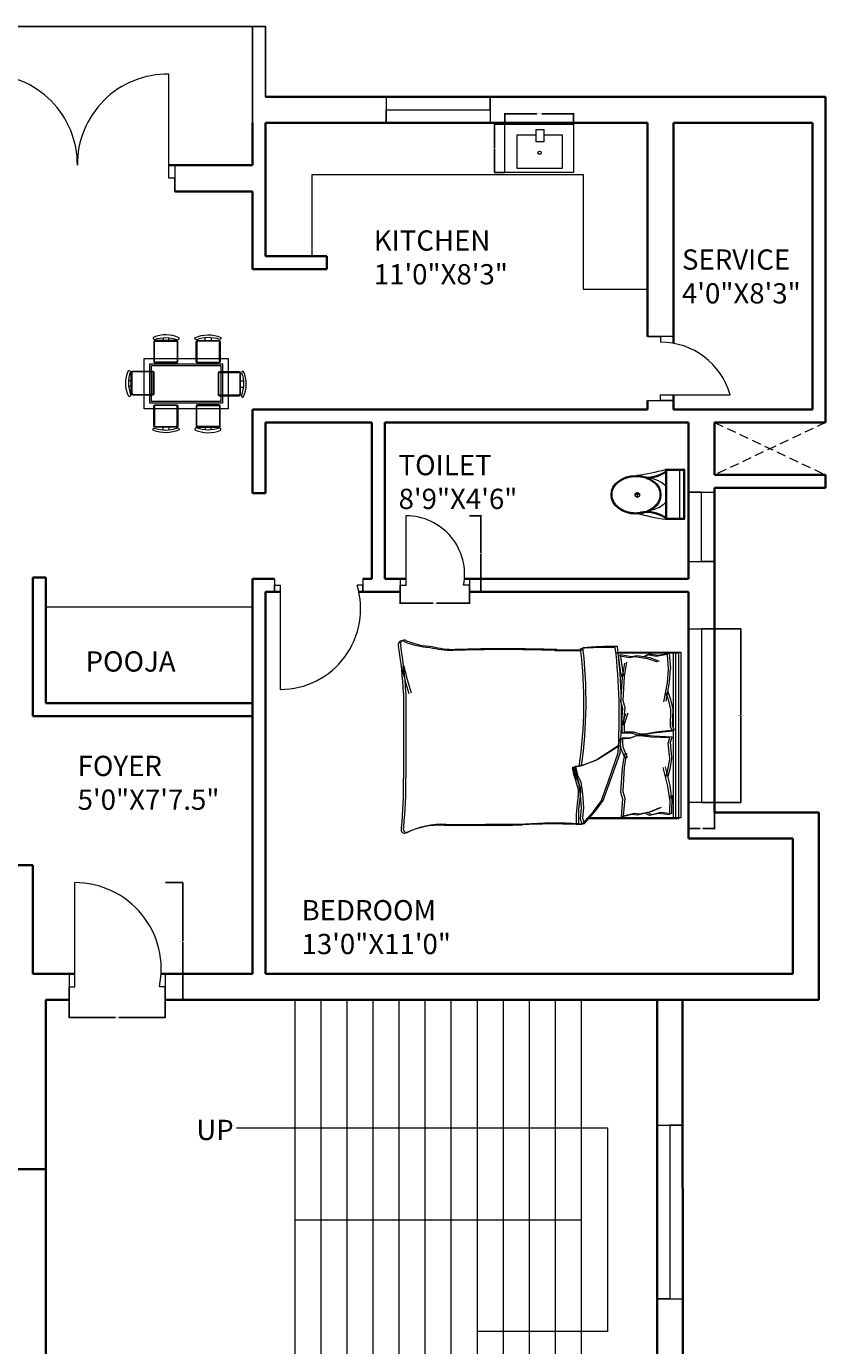
# Model space of a CAD drawing. Units: inches. Extents: x 2296 to 3812, y -1531 to 2564.
# Tile 4 of 10: x 2706 to 2983, y 1719 to 2175. Entities that reach past the tile are written whole.
import ezdxf

# ---------------------------------------------------------------- set-up
doc = ezdxf.new("R2010")
doc.units = ezdxf.units.IN
doc.linetypes.add('HIDDEN2', pattern=[4.7625, 3.175, -1.5875])
for name, color, linetype, lineweight in [('A-ANNO-DIMS', 2, 'Continuous', 18), ('A-ANNO-TEXT', 7, 'Continuous', 25), ('A-AREA-IDEN', 7, 'Continuous', 18), ('A-DOOR', 3, 'Continuous', 18), ('A-FLOR-CASE', 8, 'Continuous', 18), ('A-FLOR-FIXT', 9, 'Continuous', 18), ('A-FLOR-HRAL', 7, 'Continuous', 25), ('A-FLOR-STRS', 7, 'Continuous', 18), ('A-FURN', 8, 'Continuous', 18), ('A-GLAZ', 4, 'Continuous', 18), ('A-WALL', 7, 'Continuous', 35), ('A-WALL-HIDN', 8, 'HIDDEN2', 18)]:
    doc.layers.add(name, color=color, linetype=linetype, lineweight=lineweight)
doc.styles.get("Standard").update_dxf_attribs({"font": 'arial.ttf'})
doc.dimstyles.get("Standard").update_dxf_attribs({"dimtxt": 0.18, "dimasz": 0.18, "dimexe": 0.18, "dimexo": 0.0625, "dimgap": 0.09, "dimtad": 0, "dimtih": 1, "dimtoh": 1, "dimdec": 4, "dimzin": 0, "dimdsep": 46, "dimtxsty": 'Standard', "dimcen": 0.09, "dimadec": 0, "dimazin": 0, "dimtfac": 1, "dimtdec": 4, "dimtofl": 0, "dimtmove": 0, "dimatfit": 3, "dimfxl": 1, "dimtolj": 1, "dimtzin": 0, "dimarcsym": 0})

# ---------------------------------------------------------------- blocks, each defined once
blk = doc.blocks.new('A$C31115884')
for p, q in [((283, 498), (223, 498)), ((258, 466), (258, 523)), ((0, 200), (0, 0)), ((520, 200), (0, 200)), ((10, 190), (10, 10)), ((510, 190), (10, 190)), ((510, 10), (510, 190)), ((520, 0), (520, 200)), ((510, 54), (0, 54)), ((10, 10), (510, 10)), ((0, 0), (520, 0))]:
    blk.add_line(p, q)
blk.add_circle((256, 496), 23.6)
for centre, radius, start, end in [((2778, -205), 2807, 165.4549, 171.7133), ((-295, 403), 365, 324.2091, 9.3499), ((-295, 403), 375, 324.2091, 9.3499), ((139, 406), 293, 315.8436, 2.6563), ((806, 403), 365, 170.6501, 215.7909), ((3237, 905), 2807, 188.2867, 194.5451), ((384, 406), 293, 190.2774, 224.1564), ((806, 403), 375, 179.2036, 215.7909)]:
    blk.add_arc(centre, radius, start, end)
blk.add_ellipse((256, 510), major_axis=(0, -261), ratio=0.772727)
blk.add_open_spline([(256, 259), (263, 259), (270, 260), (288, 262), (299, 265), (320, 273), (330, 278), (350, 291), (360, 299), (378, 316), (386, 326), (402, 347), (409, 358), (421, 383), (427, 395), (436, 422), (440, 436), (445, 465), (447, 480), (448, 509), (448, 524), (445, 553), (443, 568), (436, 596), (432, 610), (422, 636), (416, 649), (402, 672), (395, 683), (379, 703), (370, 712), (351, 728), (341, 735), (321, 746), (310, 751), (289, 757), (278, 759), (256, 761), (245, 761), (223, 757), (212, 754), (191, 746), (181, 741), (161, 728), (151, 720), (133, 703), (125, 693), (110, 672), (103, 660), (90, 636), (85, 623), (76, 596), (72, 582), (67, 553), (66, 538), (64, 509), (65, 494), (68, 465), (70, 450), (77, 422), (81, 408), (91, 382), (97, 370), (111, 346), (118, 335), (135, 316), (144, 307), (162, 291), (172, 284), (193, 273), (203, 269), (225, 262), (236, 260), (250, 259), (253, 259), (256, 259)], degree=3, knots=[0, 0, 0, 0, 0.110105, 0.110105, 0.285049, 0.285049, 0.459994, 0.459994, 0.634938, 0.634938, 0.809882, 0.809882, 0.984827, 0.984827, 1.159771, 1.159771, 1.334715, 1.334715, 1.50966, 1.50966, 1.684604, 1.684604, 1.859549, 1.859549, 2.034493, 2.034493, 2.209437, 2.209437, 2.384382, 2.384382, 2.559326, 2.559326, 2.73427, 2.73427, 2.909215, 2.909215, 3.084159, 3.084159, 3.259103, 3.259103, 3.434048, 3.434048, 3.608992, 3.608992, 3.783936, 3.783936, 3.958881, 3.958881, 4.133825, 4.133825, 4.30877, 4.30877, 4.483714, 4.483714, 4.658658, 4.658658, 4.833603, 4.833603, 5.008547, 5.008547, 5.183491, 5.183491, 5.358436, 5.358436, 5.53338, 5.53338, 5.708324, 5.708324, 5.883269, 5.883269, 6.058213, 6.058213, 6.233158, 6.233158, 6.283185, 6.283185, 6.283185, 6.283185])
blk = doc.blocks.new('DOOR-SERVICE-24-NE')
for p, q in [((9, 22.16), (0, 22.16)), ((0, 22.16), (4.5, 22.16)), ((4.5, 22.16), (4.5, 20.16)), ((0, 0), (9, 0)), ((4.5, 0), (4.5, 2)), ((4.5, 2), (28.5, 2)), ((9, 0), (4.5, 0))]:
    blk.add_line(p, q)
blk.add_arc((4.5, -4.78), 24.94, 15.78, 90)
blk = doc.blocks.new('DOOR-BALCONY-PAIR-N')
for p, q in [((2, 4.5), (2, 40.5)), ((64.91, 4.5), (64.91, 40.5)), ((0, 9), (0, 0)), ((66.91, 9), (66.91, 0)), ((0, 0), (0, 4.5)), ((0, 4.5), (2, 4.5)), ((66.91, 4.5), (64.91, 4.5)), ((66.91, 0), (66.91, 4.5))]:
    blk.add_line(p, q)
for centre, radius, start, end in [((2, 9.22), 31.28, 359.5901, 90), ((64.41, 9.36), 31.14, 89.0831, 180.6679)]:
    blk.add_arc(centre, radius, start, end)
blk = doc.blocks.new('DOOR-BEDROOM-36-NE')
for p, q in [((0, 38.25), (0, 33.75)), ((30.56, 38.25), (30.56, 33.75)), ((0, 33.75), (0, 36)), ((0, 36), (0, 36)), ((0, 36), (2, 36)), ((2, 36), (2, 0)), ((30.56, 36), (28.56, 36)), ((30.56, 33.75), (30.56, 36))]:
    blk.add_line(p, q)
blk.add_arc((2, 27.8), 27.8, 270, 17.157)
blk = doc.blocks.new('DOOR-BATH-24-NE')
for p, q in [((2, 2.25), (2, 26.25)), ((0, 4.5), (0, 0)), ((0, 0), (0, 2.25)), ((0, 2.25), (2, 2.25)), ((23.89, 2.25), (21.89, 2.25)), ((23.89, 4.5), (23.89, 0)), ((23.89, 0), (23.89, 2.25))]:
    blk.add_line(p, q)
blk.add_arc((2, 6.01), 20.24, 349.2884, 90)
blk = doc.blocks.new('DOOR-ENTRY-36-N')
for p, q in [((2, 4.5), (2, 40.5)), ((0, 9), (0, 0)), ((33.22, 9), (33.22, 0)), ((0, 0), (0, 4.5)), ((0, 4.5), (2, 4.5)), ((33.22, 4.5), (31.22, 4.5)), ((33.22, 0), (33.22, 4.5))]:
    blk.add_line(p, q)
blk.add_arc((2, 10.64), 29.86, 348.1386, 90)
blk = doc.blocks.new('WIN-36-KITCHEN')
for p, q in [((0, 9), (0, 0)), ((36, 4.5), (36, 9)), ((36, 9), (36, 0)), ((0, 0), (0, 4.5)), ((0, 4.5), (36, 4.5))]:
    blk.add_line(p, q)
blk = doc.blocks.new('WIN-24-BATH')
for p, q in [((4.5, 24), (0, 24)), ((0, 24), (9, 24)), ((4.5, 0), (4.5, 24)), ((0, 0), (9, 0)), ((9, 0), (4.5, 0))]:
    blk.add_line(p, q)
blk = doc.blocks.new('WIN-60-JAMB-A')
for p, q in [((0, 60), (9, 60)), ((9, 60), (4.5, 60)), ((4.5, 60), (4.5, 0)), ((9, 0), (0, 0)), ((4.5, 0), (9, 0))]:
    blk.add_line(p, q)
blk = doc.blocks.new('WIN-60-STAIR')
for p, q in [((0, 59.99), (8.73, 60.01)), ((8.73, 60.01), (4.36, 60)), ((4.36, 60), (4.36, 0)), ((0, 0), (8.81, 0.01)), ((4.36, 0), (0, 0))]:
    blk.add_line(p, q)
blk = doc.blocks.new('BED-DOUBLE')
for p, q in [((48.49, 95), (18.98, 95)), ((3.07, 35.36), (3.17, 33.26, 4.64)), ((5.01, 34.01), (3.17, 33.26)), ((3.17, 33.26), (7.61, 29.37)), ((8.72, 33.63), (5.01, 34.01)), ((13.37, 34.01), (8.72, 33.63)), ((17.45, 34.56), (13.37, 34.01)), ((19.86, 35.68), (17.45, 34.56)), ((22.83, 36.42), (19.86, 35.68)), ((23.21, 34.01), (22.83, 36.42)), ((25.25, 28.62), (23.21, 34.01)), ((5.09, 0), (5.09, 31.9)), ((7.61, 29.37), (11.14, 26.77)), ((30.27, 20.84), (25.25, 28.62)), ((11.14, 26.77), (17.82, 24.36)), ((17.82, 24.36), (27.82, 20.84)), ((11.92, 19.38), (5.77, 19.87)), ((5.77, 19.87), (6.7, 16.11)), ((14.27, 20.05), (11.92, 19.38)), ((22.67, 19.54), (14.27, 20.05)), ((27.51, 18.74), (22.67, 19.54)), ((29.68, 20.07), (26, 18.53)), ((32.62, 20.25), (29.68, 20.07)), ((32.82, 17.04), (32.62, 20.25)), ((34.71, 16.28), (34.71, 19.5)), ((34.71, 19.5), (37.65, 19.5)), ((43.31, 19.38), (37.16, 19.87)), ((37.65, 19.5), (41.42, 18.19)), ((45.66, 20.05), (43.31, 19.38)), ((54.06, 19.54), (45.66, 20.05)), ((54.06, 19.54), (55.42, 19.92)), ((58.9, 18.74), (54.06, 19.54)), ((55.42, 19.92), (61.53, 20.79)), ((61.53, 20.79), (60.84, 16.98)), ((62.38, 21.71), (62.38, 0)), ((6.7, 16.11), (6.47, 14.18)), ((6.47, 14.18), (7.43, 9.9)), ((33.66, 14.84), (32.82, 17.04)), ((33.75, 13.28), (33.66, 14.84)), ((34.01, 14.03), (34.71, 16.28)), ((34.01, 12.47), (34.01, 14.03)), ((61.19, 15.07), (60.49, 10.74)), ((60.84, 16.98), (61.19, 15.07)), ((6.21, 10), (6.83, 11.25)), ((6.93, 6.92), (6.21, 10)), ((7.43, 9.9), (8.85, 6.69)), ((33.01, 2.99), (33.3, 9.43)), ((33.3, 9.43), (33.75, 13.28)), ((34.71, 8.66), (34.01, 12.47)), ((60.49, 10.74), (59.28, 7.44)), ((61.71, 10.91), (61.01, 12.12)), ((61.19, 7.79), (61.71, 10.91)), ((6.47, 3.07), (6.93, 6.92)), ((16.3, 3.68), (22.8, 5.3)), ((35.4, 2.24), (34.71, 8.66)), ((52.03, 3.98), (45.45, 5.19)), ((61.88, 3.98), (61.19, 7.79)), ((62.38, 1.84), (5.09, 1.84)), ((62.38, 0), (5.09, 0)), ((6.47, 3.07), (12.95, 2.95)), ((11.75, 3.05), (16.3, 3.68)), ((12.95, 2.95), (11.75, 3.05)), ((19.55, 4.4), (22.03, 3.69)), ((22.03, 3.69), (25.54, 3.04)), ((25.54, 3.04), (25.93, 3.07)), ((25.93, 3.07), (31.24, 3.57)), ((31.24, 3.57), (33.01, 2.99)), ((37.13, 2.94), (35.4, 2.24)), ((42.46, 2.76), (37.13, 2.94)), ((42.85, 2.76), (42.46, 2.76)), ((46.31, 3.63), (42.85, 2.76)), ((48.74, 4.5), (46.31, 3.63)), ((56.62, 3.63), (52.03, 3.98)), ((56.74, 3.61), (56.62, 3.63)), ((61.87, 4), (56.74, 3.61))]:
    blk.add_line(p, q)
for centre, radius, start, end in [((1.32, 94.55), 1.32, 62.6588, 176.02), ((87.19, -28.43), 127.63, 103.3832, 107.7053), ((40.86, 240.78), 145.97, 272.9958, 279.4091), ((65.24, 95.57), 1.31, 326.1736, 113.4781), ((-24.75, 82.32), 27.65, 357.4714, 26.4681), ((17.21, 254.49), 159.5, 264.4998, 270.6351), ((92.52, 84.25), 28.25, 157.9751, 176.652), ((98.8, 77.34), 35.53, 166.0648, 178.9113), ((5471.89, 81.31), 5469.02, 180.00217, 180.28689), ((-514.68, 60.68), 578.22, 358.22771, 1.71854), ((-151.96, 43.54), 155.25, 356.9791, 3.8365), ((267.13, 37.37), 203.94, 178.4762, 181.0082), ((29.2, 1.78), 35.55, 100.6617, 109.8806), ((22.63, 36.49), 0.221, 340.2464, 91.1377), ((5.01, -7.98), 43.38, 79.8763, 92.5657), ((14.11, 42.04), 7.46, 258.6608, 293.7384), ((45.26, 187.4), 154.68, 261.7845, 276.9006), ((-35.55, 24.09), 99.87, 358.7218, 5.604), ((40.94, 218.26), 197.77, 266.0865, 276.7821)]:
    blk.add_arc(centre, radius, start, end)
blk = doc.blocks.new('SINK-KITCHEN')
for points in [[(0, 16.77), (23.71, 16.77), (23.71, 0), (0, 0)], [(10.76, 14.92), (13.44, 14.92), (13.44, 10.63), (10.76, 10.63)]]:
    blk.add_lwpolyline(points, close=True)
blk.add_lwpolyline([(13.44, 13.06), (19.73, 13.06), (19.73, 1.48), (4.23, 1.48), (4.23, 13.06), (10.76, 13.06)])
blk.add_circle((11.97, 6.87), 0.556)
blk = doc.blocks.new('STAIR-DOGLEG')
for p, q in [((20.27, 0), (20.27, 152.06)), ((29.27, 0), (29.27, 152.06)), ((38.27, 0), (38.27, 152.06)), ((47.27, 0), (47.27, 152.06)), ((56.27, 0), (56.27, 152.06)), ((65.27, 0), (65.27, 152.06)), ((74.27, 0), (74.27, 152.06)), ((83.27, 0), (83.27, 152.06)), ((92.27, 0), (92.27, 152.06)), ((101.27, 0), (101.27, 152.06)), ((110.27, 0), (110.27, 152.06)), ((119.27, 0), (119.27, 152.06)), ((0, 107.85), (128.27, 107.85)), ((128.27, 107.85), (128.27, 37.4)), ((20.27, 76.03), (119.27, 76.03)), ((128.27, 37.4), (83.27, 37.4))]:
    blk.add_line(p, q)
blk = doc.blocks.new('COUNTER-KITCHEN-N')
for p, q in [((0, 11.4), (0, 39.66)), ((0, 39.66), (93.66, 39.66)), ((93.66, 39.66), (93.66, 0)), ((93.66, 0), (115.91, 0))]:
    blk.add_line(p, q)
blk = doc.blocks.new('*D47')
at = {"layer": 'A-ANNO-DIMS', "color": 0, "lineweight": -2, "transparency": 16777216}
for p, q in [((2871.76, 2141.32), (2871.76, 2144.99)), ((2871.94, 2144.81), (2882.76, 2144.81)), ((2895.29, 2144.81), (2884.47, 2144.81)), ((2895.47, 2141.32), (2895.47, 2144.99))]:
    blk.add_line(p, q, dxfattribs=at)
at = {"layer": 'A-ANNO-DIMS', "color": 0, "transparency": 16777216}
for points in [[(2871.94, 2144.84), (2871.94, 2144.78), (2871.76, 2144.81)], [(2895.29, 2144.84), (2895.29, 2144.78), (2895.47, 2144.81)]]:
    blk.add_solid(points, dxfattribs=at)
at = {"layer": 'Defpoints', "color": 0, "transparency": 16777216}
for p in [(2895.47, 2144.81), (2871.76, 2141.25), (2895.47, 2141.25)]:
    blk.add_point(p, dxfattribs=at)
at = {"layer": 'A-ANNO-DIMS', "color": 0, "transparency": 16777216, "insert": (2883.61, 2144.81), "char_height": 0.18, "attachment_point": 5}
blk.add_mtext('\\A1;SINK 24 TYP.', dxfattribs=at)
blk = doc.blocks.new('*D48')
at = {"layer": 'A-ANNO-DIMS', "color": 0, "lineweight": -2, "transparency": 16777216}
for p, q in [((2871.7, 2141.25), (2868.02, 2141.25)), ((2868.2, 2141.07), (2868.2, 2133.05)), ((2868.2, 2124.66), (2868.2, 2132.69)), ((2871.7, 2124.48), (2868.02, 2124.48))]:
    blk.add_line(p, q, dxfattribs=at)
at = {"layer": 'A-ANNO-DIMS', "color": 0, "transparency": 16777216}
for points in [[(2868.17, 2141.07), (2868.23, 2141.07), (2868.2, 2141.25)], [(2868.17, 2124.66), (2868.23, 2124.66), (2868.2, 2124.48)]]:
    blk.add_solid(points, dxfattribs=at)
at = {"layer": 'Defpoints', "color": 0, "transparency": 16777216}
for p in [(2868.2, 2141.25), (2871.76, 2141.25), (2871.76, 2124.48)]:
    blk.add_point(p, dxfattribs=at)
at = {"layer": 'A-ANNO-DIMS', "color": 0, "transparency": 16777216, "insert": (2868.2, 2132.87), "char_height": 0.18, "attachment_point": 5}
blk.add_mtext('\\A1;17 TYP.', dxfattribs=at)
blk = doc.blocks.new('*D67')
at = {"layer": 'A-ANNO-DIMS', "color": 0, "lineweight": -2, "transparency": 16777216}
for p, q in [((2859.56, 2005.91), (2863.62, 2005.91)), ((2863.44, 2005.73), (2863.44, 1992.97)), ((2863.44, 1979.84), (2863.44, 1992.6)), ((2859.56, 1979.66), (2863.62, 1979.66))]:
    blk.add_line(p, q, dxfattribs=at)
at = {"layer": 'A-ANNO-DIMS', "color": 0, "transparency": 16777216}
for points in [[(2863.41, 2005.73), (2863.47, 2005.73), (2863.44, 2005.91)], [(2863.41, 1979.84), (2863.47, 1979.84), (2863.44, 1979.66)]]:
    blk.add_solid(points, dxfattribs=at)
at = {"layer": 'Defpoints', "color": 0, "transparency": 16777216}
for p in [(2859.5, 2005.91), (2863.44, 2005.91), (2859.5, 1979.66)]:
    blk.add_point(p, dxfattribs=at)
at = {"layer": 'A-ANNO-DIMS', "color": 0, "transparency": 16777216, "insert": (2863.44, 1992.78), "char_height": 0.18, "attachment_point": 5}
blk.add_mtext('\\A1;BATH DOOR 26 TYP.', dxfattribs=at)
blk = doc.blocks.new('*D68')
at = {"layer": 'A-ANNO-DIMS', "color": 0, "lineweight": -2, "transparency": 16777216}
for p, q in [((2835.61, 1979.6), (2835.61, 1975.54)), ((2859.5, 1979.6), (2859.5, 1975.54)), ((2835.79, 1975.72), (2847.03, 1975.72)), ((2859.32, 1975.72), (2848.09, 1975.72))]:
    blk.add_line(p, q, dxfattribs=at)
at = {"layer": 'A-ANNO-DIMS', "color": 0, "transparency": 16777216}
for points in [[(2835.79, 1975.75), (2835.79, 1975.69), (2835.61, 1975.72)], [(2859.32, 1975.75), (2859.32, 1975.69), (2859.5, 1975.72)]]:
    blk.add_solid(points, dxfattribs=at)
at = {"layer": 'Defpoints', "color": 0, "transparency": 16777216}
for p in [(2835.61, 1979.66), (2859.5, 1979.66), (2859.5, 1975.72)]:
    blk.add_point(p, dxfattribs=at)
at = {"layer": 'A-ANNO-DIMS', "color": 0, "transparency": 16777216, "insert": (2847.56, 1975.72), "char_height": 0.18, "attachment_point": 5}
blk.add_mtext('\\A1;24 TYP.', dxfattribs=at)
blk = doc.blocks.new('*D73')
at = {"layer": 'A-ANNO-DIMS', "color": 0, "lineweight": -2, "transparency": 16777216}
for p, q in [((2754.46, 1879.16), (2760.65, 1879.16)), ((2760.47, 1878.98), (2760.47, 1859.09)), ((2760.47, 1838.84), (2760.47, 1858.72)), ((2754.46, 1838.66), (2760.65, 1838.66))]:
    blk.add_line(p, q, dxfattribs=at)
at = {"layer": 'A-ANNO-DIMS', "color": 0, "transparency": 16777216}
for points in [[(2760.44, 1878.98), (2760.5, 1878.98), (2760.47, 1879.16)], [(2760.44, 1838.84), (2760.5, 1838.84), (2760.47, 1838.66)]]:
    blk.add_solid(points, dxfattribs=at)
at = {"layer": 'Defpoints', "color": 0, "transparency": 16777216}
for p in [(2754.39, 1879.16), (2760.47, 1879.16), (2754.39, 1838.66)]:
    blk.add_point(p, dxfattribs=at)
at = {"layer": 'A-ANNO-DIMS', "color": 0, "transparency": 16777216, "insert": (2760.47, 1858.91), "char_height": 0.18, "attachment_point": 5}
blk.add_mtext('\\A1;ENTRY DOOR 41 TYP.', dxfattribs=at)
blk = doc.blocks.new('*D74')
at = {"layer": 'A-ANNO-DIMS', "color": 0, "lineweight": -2, "transparency": 16777216}
for p, q in [((2721.17, 1838.6), (2721.17, 1832.4)), ((2754.39, 1838.6), (2754.39, 1832.4)), ((2721.35, 1832.58), (2737.25, 1832.58)), ((2754.21, 1832.58), (2738.31, 1832.58))]:
    blk.add_line(p, q, dxfattribs=at)
at = {"layer": 'A-ANNO-DIMS', "color": 0, "transparency": 16777216}
for points in [[(2721.35, 1832.61), (2721.35, 1832.55), (2721.17, 1832.58)], [(2754.21, 1832.61), (2754.21, 1832.55), (2754.39, 1832.58)]]:
    blk.add_solid(points, dxfattribs=at)
at = {"layer": 'Defpoints', "color": 0, "transparency": 16777216}
for p in [(2721.17, 1838.66), (2754.39, 1838.66), (2754.39, 1832.58)]:
    blk.add_point(p, dxfattribs=at)
at = {"layer": 'A-ANNO-DIMS', "color": 0, "transparency": 16777216, "insert": (2737.78, 1832.58), "char_height": 0.18, "attachment_point": 5}
blk.add_mtext('\\A1;33 TYP.', dxfattribs=at)
blk = doc.blocks.new('*D95')
at = {"layer": 'A-ANNO-DIMS', "color": 0, "lineweight": -2, "transparency": 16777216}
for p, q in [((2944.29, 1966.83), (2953.41, 1966.83)), ((2953.23, 1966.65), (2953.23, 1937.01)), ((2953.23, 1907.01), (2953.23, 1936.65)), ((2944.29, 1906.83), (2953.41, 1906.83))]:
    blk.add_line(p, q, dxfattribs=at)
at = {"layer": 'A-ANNO-DIMS', "color": 0, "transparency": 16777216}
for points in [[(2953.2, 1966.65), (2953.26, 1966.65), (2953.23, 1966.83)], [(2953.2, 1907.01), (2953.26, 1907.01), (2953.23, 1906.83)]]:
    blk.add_solid(points, dxfattribs=at)
at = {"layer": 'Defpoints', "color": 0, "transparency": 16777216}
for p in [(2944.23, 1966.83), (2953.23, 1966.83), (2944.23, 1906.83)]:
    blk.add_point(p, dxfattribs=at)
at = {"layer": 'A-ANNO-DIMS', "color": 0, "transparency": 16777216, "insert": (2953.23, 1936.83), "char_height": 0.18, "attachment_point": 5}
blk.add_mtext('\\A1;WINDOW 60 TYP.', dxfattribs=at)
blk = doc.blocks.new('*D96')
at = {"layer": 'A-ANNO-DIMS', "color": 0, "lineweight": -2, "transparency": 16777216}
for p, q in [((2935.23, 1906.77), (2935.23, 1897.65)), ((2944.23, 1906.77), (2944.23, 1897.65)), ((2935.41, 1897.83), (2939.27, 1897.83)), ((2944.05, 1897.83), (2940.19, 1897.83))]:
    blk.add_line(p, q, dxfattribs=at)
at = {"layer": 'A-ANNO-DIMS', "color": 0, "transparency": 16777216}
for points in [[(2935.41, 1897.86), (2935.41, 1897.8), (2935.23, 1897.83)], [(2944.05, 1897.86), (2944.05, 1897.8), (2944.23, 1897.83)]]:
    blk.add_solid(points, dxfattribs=at)
at = {"layer": 'Defpoints', "color": 0, "transparency": 16777216}
for p in [(2935.23, 1906.83), (2944.23, 1906.83), (2944.23, 1897.83)]:
    blk.add_point(p, dxfattribs=at)
at = {"layer": 'A-ANNO-DIMS', "color": 0, "transparency": 16777216, "insert": (2939.73, 1897.83), "char_height": 0.18, "attachment_point": 5}
blk.add_mtext('\\A1;9 TYP.', dxfattribs=at)

msp = doc.modelspace()

# ---------------------------------------------------------------- linework, layer by layer
at = {"layer": 'A-FLOR-CASE'}
msp.add_line((2784.5693, 1974.3293), (2713.1754, 1974.3293), dxfattribs=at)
at = {"layer": 'A-FLOR-HRAL'}
for p, q in [((2789.0693, 2175.0276), (2655.5693, 2175.0276)), ((2660.0693, 2175.0276), (2789.0693, 2175.0276)), ((2784.5693, 2141.6578), (2784.5693, 2175.0276)), ((2789.0693, 2175.0276), (2789.0693, 2150.6578))]:
    msp.add_line(p, q, dxfattribs=at)
at = {"layer": 'A-FURN'}
for points in [[(2750.6939, 2066.831, -0.17580919), (2758.5956, 2066.7712, 0.57839206), (2759.1942, 2067.4294, 0.21452438), (2750.2749, 2067.5491, 0.55201397), (2750.6939, 2066.831, -0.06507904)], [(2758.2603, 2066.5139), (2750.9247, 2066.5139, 0.41421356), (2750.4115, 2066.0007), (2750.4115, 2059.2556, 0.41421356), (2750.9247, 2058.7424), (2758.2603, 2058.7424, 0.41421356), (2758.7736, 2059.2556), (2758.7736, 2066.0007, 0.41421356), (2758.2603, 2066.5139)], [(2755.6837, 2066.5139), (2755.6837, 2067.4416, -0.06475861)], [(2765.2478, 2066.7712, -0.57839206), (2764.6492, 2067.4294, -0.21452438), (2773.5685, 2067.5491, -0.55201397), (2773.1495, 2066.831, 0.1758092), (2765.2478, 2066.7712)], [(2772.9187, 2066.5139, -0.41421356), (2773.4319, 2066.0007), (2773.4319, 2059.2556, -0.41421356), (2772.9187, 2058.7424), (2765.583, 2058.7424, -0.41421356), (2765.0698, 2059.2556), (2765.0698, 2066.0007, -0.41421356), (2765.583, 2066.5139), (2772.9187, 2066.5139)], [(2768.1597, 2066.5139), (2768.1597, 2067.4416, 0.06475861)], [(2742.4272, 2047.7496, -0.57839206), (2741.769, 2047.151, -0.21452438), (2741.6493, 2056.0703, -0.55201397), (2742.3673, 2055.6513, 0.17580937), (2742.4272, 2047.7496)], [(2742.6845, 2055.4205, -0.41421356), (2743.1977, 2055.9337), (2749.9427, 2055.9337, -0.41421356), (2750.4559, 2055.4205), (2750.4559, 2048.0848, -0.41421356), (2749.9427, 2047.5716), (2743.1977, 2047.5716, -0.41421356), (2742.6845, 2048.0848), (2742.6845, 2055.4205)], [(2780.4598, 2055.1693, 0.41421356), (2779.9466, 2055.6825), (2773.2015, 2055.6825, 0.41421356), (2772.6883, 2055.1693), (2772.6883, 2047.8336, 0.41421356), (2773.2015, 2047.3204), (2779.9466, 2047.3204, 0.41421356), (2780.4598, 2047.8336), (2780.4598, 2055.1693)], [(2780.7769, 2055.4001, -0.17580919), (2780.7171, 2047.4984, 0.57839206), (2781.3753, 2046.8997, 0.21452438), (2781.495, 2055.8191, 0.55201397), (2780.7769, 2055.4001, -0.06507904)], [(2742.6845, 2050.6615), (2741.7567, 2050.6615, 0.06475861)], [(2780.4598, 2050.4103), (2781.3875, 2050.4103, -0.06475861)], [(2758.2603, 2036.5306), (2750.9247, 2036.5306, -0.41421356), (2750.4115, 2037.0439), (2750.4115, 2043.7889, -0.41421356), (2750.9247, 2044.3021), (2758.2603, 2044.3021, -0.41421356), (2758.7736, 2043.7889), (2758.7736, 2037.0439, -0.41421356), (2758.2603, 2036.5306)], [(2772.9187, 2036.5306, 0.41421356), (2773.4319, 2037.0439), (2773.4319, 2043.7889, 0.41421356), (2772.9187, 2044.3021), (2765.583, 2044.3021, 0.41421356), (2765.0698, 2043.7889), (2765.0698, 2037.0439, 0.41421356), (2765.583, 2036.5306), (2772.9187, 2036.5306)], [(2758.5956, 2036.2733, -0.57839206), (2759.1942, 2035.6151, -0.21452438), (2750.2749, 2035.4954, -0.55201397), (2750.6939, 2036.2135, 0.17580929), (2758.5956, 2036.2733)], [(2755.6837, 2036.5306), (2755.6837, 2035.6029, 0.06475861)], [(2773.1495, 2036.2135, -0.17580928), (2765.2478, 2036.2733, 0.57839206), (2764.6492, 2035.6151, 0.21452438), (2773.5685, 2035.4954, 0.55201397), (2773.1495, 2036.2135, -0.06507904)], [(2768.1597, 2036.5306), (2768.1597, 2035.6029, -0.06475861)]]:
    msp.add_lwpolyline(points, format="xyb", dxfattribs=at)
for points in [[(2750.9278, 2066.2827), (2758.0291, 2066.2827, -0.41421356), (2758.5424, 2065.7694), (2758.5424, 2059.4868, -0.41421356), (2758.0291, 2058.9736), (2750.9278, 2058.9736, -0.51206948), (2750.6427, 2059.4868), (2750.6427, 2065.7694, -0.51206948)], [(2772.9156, 2066.2827), (2765.8142, 2066.2827, 0.41421356), (2765.301, 2065.7694), (2765.301, 2059.4868, 0.41421356), (2765.8142, 2058.9736), (2772.9156, 2058.9736, 0.51206948), (2773.2007, 2059.4868), (2773.2007, 2065.7694, 0.51206948)], [(2742.9157, 2055.4174), (2742.9157, 2048.316, 0.41421356), (2743.4289, 2047.8028), (2749.7115, 2047.8028, 0.41421356), (2750.2247, 2048.316), (2750.2247, 2055.4174, 0.51206948), (2749.7115, 2055.7025), (2743.4289, 2055.7025, 0.51206948)], [(2780.2286, 2055.1662), (2780.2286, 2048.0648, -0.41421356), (2779.7154, 2047.5516), (2773.4328, 2047.5516, -0.41421356), (2772.9195, 2048.0648), (2772.9195, 2055.1662, -0.51206948), (2773.4328, 2055.4513), (2779.7154, 2055.4513, -0.51206948)], [(2750.9278, 2036.7618), (2758.0291, 2036.7618, 0.41421356), (2758.5424, 2037.2751), (2758.5424, 2043.5577, 0.41421356), (2758.0291, 2044.0709), (2750.9278, 2044.0709, 0.51206948), (2750.6427, 2043.5577), (2750.6427, 2037.2751, 0.51206948)], [(2772.9156, 2036.7618), (2765.8142, 2036.7618, -0.41421356), (2765.301, 2037.2751), (2765.301, 2043.5577, -0.41421356), (2765.8142, 2044.0709), (2772.9156, 2044.0709, -0.51206948), (2773.2007, 2043.5577), (2773.2007, 2037.2751, -0.51206948)]]:
    msp.add_lwpolyline(points, format="xyb", close=True, dxfattribs=at)
for points in [[(2753.6303, 2067.4585), (2753.6303, 2066.5139)], [(2770.2131, 2067.4585), (2770.2131, 2066.5139)], [(2741.7399, 2052.7148), (2742.6845, 2052.7148)], [(2781.4044, 2052.4636), (2780.4598, 2052.4636)], [(2753.6303, 2035.586), (2753.6303, 2036.5306)], [(2770.2131, 2035.586), (2770.2131, 2036.5306)]]:
    msp.add_lwpolyline(points, dxfattribs=at)
for points in [[(2747.1055, 2060.3187), (2776.1163, 2060.3187), (2776.1163, 2042.9123), (2747.1055, 2042.9123)], [(2749.0396, 2058.3847), (2774.1822, 2058.3847), (2774.1822, 2044.8463), (2749.0396, 2044.8463)], [(2749.6198, 2057.8044), (2773.602, 2057.8044), (2773.602, 2045.4265), (2749.6198, 2045.4265)]]:
    msp.add_lwpolyline(points, close=True, dxfattribs=at)
at = {"layer": 'A-WALL'}
for p, q in [((2789.0693, 2150.6578), (2982.5693, 2150.6578)), ((2789.0693, 2150.6578), (2982.5693, 2150.6578)), ((2982.5693, 2150.6578), (2982.5693, 2038.1578)), ((2784.5693, 2141.6578), (2784.5693, 2127.0276)), ((2789.0693, 2141.6578), (2789.0693, 2095.613)), ((2789.0693, 2141.6578), (2921.0693, 2141.6578)), ((2921.0693, 2141.6578), (2921.0693, 2067.9121)), ((2930.0693, 2141.6578), (2930.0693, 2065.5027)), ((2930.0693, 2141.6578), (2978.0693, 2141.6578)), ((2978.0693, 2141.6578), (2978.0693, 2042.6578)), ((2755.6832, 2127.0276), (2784.5693, 2127.0276)), ((2784.5693, 2118.0276), (2757.6832, 2118.0276)), ((2784.5693, 2118.0276), (2784.5693, 2091.113)), ((2810.2513, 2095.613), (2789.0693, 2095.613)), ((2810.2513, 2091.113), (2810.2513, 2095.613)), ((2784.5693, 2091.113), (2810.2513, 2091.113)), ((2930.0693, 2047.7544), (2930.0693, 2042.6578)), ((2789.0693, 2042.6578), (2784.5693, 2042.6578)), ((2784.5693, 2042.6578), (2784.5693, 2013.7336)), ((2789.0693, 2042.6578), (2921.0693, 2042.6578)), ((2921.0693, 2045.7544), (2921.0693, 2042.6578)), ((2930.0693, 2042.6578), (2978.0693, 2042.6578)), ((2930.0693, 2042.6578), (2978.0693, 2042.6578)), ((2789.0693, 2038.1578), (2825.7282, 2038.1578)), ((2789.0693, 2038.1578), (2789.0693, 2013.7336)), ((2825.7282, 2038.1578), (2825.7282, 1984.1578)), ((2830.2282, 1984.1578), (2830.2282, 2038.1578)), ((2830.2282, 2038.1578), (2935.2282, 2038.1578)), ((2830.2282, 2038.1578), (2935.2282, 2038.1578)), ((2935.2282, 2038.1578), (2935.2282, 1984.1578)), ((2944.2282, 2038.1578), (2982.5693, 2038.1578)), ((2944.2282, 2020.0533), (2944.2282, 2038.1578)), ((2944.2282, 2020.0533), (2982.5693, 2020.0533)), ((2982.5693, 2020.0533), (2982.5693, 2015.5533)), ((2982.5693, 2020.0533), (2982.5693, 2015.5533)), ((2982.5693, 2015.5533), (2944.2282, 2015.5533)), ((2944.2282, 1990.1003), (2944.2282, 2015.5533)), ((2789.0693, 2013.7336), (2784.5693, 2013.7336)), ((2944.2282, 2011.1578), (2944.2282, 2011.1578)), ((2944.2282, 1984.1578), (2944.2282, 2006.6578)), ((2708.6754, 1984.5954), (2708.6754, 1936.6578)), ((2708.6754, 1936.6578), (2708.6754, 1984.5954)), ((2708.6754, 1984.5954), (2713.1754, 1984.5954)), ((2713.1754, 1984.5954), (2713.1754, 1941.1578)), ((2789.0693, 1984.1578), (2784.5693, 1984.1578)), ((2784.5693, 1984.1578), (2784.5693, 1979.704)), ((2784.5693, 1984.1578), (2784.5693, 1847.6578)), ((2789.0693, 1984.1578), (2792.1173, 1984.1578)), ((2822.6796, 1984.1578), (2825.7282, 1984.1578)), ((2830.2282, 1984.1578), (2837.6148, 1984.1578)), ((2857.7967, 1984.1578), (2935.2282, 1984.1578)), ((2944.2282, 1903.3996), (2944.2282, 1984.1578)), ((2789.0693, 1979.6578), (2794.1173, 1979.6578)), ((2789.0693, 1979.6578), (2789.0693, 1847.6578)), ((2821.2724, 1979.6578), (2835.6148, 1979.6578)), ((2859.5006, 1979.6578), (2935.2282, 1979.6578)), ((2935.2282, 1979.6578), (2935.2282, 1894.3996)), ((2713.1754, 1941.1578), (2784.5693, 1941.1578)), ((2784.5693, 1936.6578), (2708.6754, 1936.6578)), ((2784.5693, 1847.6578), (2784.5693, 1936.6578)), ((2980.2282, 1903.3996), (2944.2282, 1903.3996)), ((2980.2282, 1894.3996), (2980.2282, 1903.3996)), ((2944.2282, 1894.3996), (2935.2282, 1894.3996)), ((2971.2282, 1894.3996), (2944.2282, 1894.3996)), ((2971.2282, 1847.6578), (2971.2282, 1894.3996)), ((2980.2282, 1838.6578), (2980.2282, 1894.3996)), ((2624.0585, 1885.1578), (2708.6754, 1885.1578)), ((2708.6754, 1880.6578), (2708.6754, 1885.1578)), ((2708.6754, 1880.6578), (2708.6754, 1847.6578)), ((2708.6754, 1847.6578), (2713.1754, 1847.6578)), ((2713.1754, 1847.6578), (2723.1698, 1847.6578)), ((2713.1754, 1847.6578), (2723.1698, 1847.6578)), ((2752.9868, 1847.6578), (2784.5693, 1847.6578)), ((2752.9868, 1847.6578), (2784.5693, 1847.6578)), ((2789.0693, 1847.6578), (2935.2282, 1847.6578)), ((2789.0693, 1847.6578), (2935.2282, 1847.6578)), ((2944.2282, 1847.6578), (2935.2282, 1847.6578)), ((2944.2282, 1847.6578), (2959.2282, 1847.6578)), ((2959.2282, 1847.6578), (2971.2282, 1847.6578)), ((2713.1754, 1838.6578), (2721.1698, 1838.6578)), ((2713.1754, 1838.6578), (2713.1754, 1789.1578)), ((2713.1754, 1838.6578), (2713.1754, 1780.1578)), ((2754.3941, 1838.6578), (2789.0693, 1838.6578)), ((2789.0693, 1838.6578), (2944.2282, 1838.6578)), ((2789.0693, 1838.6578), (2933.0693, 1838.6578)), ((2924.405, 1686.6012), (2924.405, 1838.6578)), ((2933.0693, 1838.6578), (2933.405, 1605.6012)), ((2935.2282, 1838.6578), (2944.2282, 1838.6578)), ((2944.2282, 1838.6578), (2971.2282, 1838.6578)), ((2971.2282, 1838.6578), (2980.2282, 1838.6578)), ((2638.4, 1780.1578), (2713.1754, 1780.1578)), ((2713.1754, 1780.1578), (2713.1754, 1674.9485))]:
    msp.add_line(p, q, dxfattribs=at)
at = {"layer": 'A-WALL-HIDN'}
for p, q in [((2982.5693, 2038.1578), (2944.2282, 2020.0533)), ((2944.2282, 2038.1578), (2982.5693, 2020.0533)), ((2982.5693, 2020.0533), (2982.5693, 2020.0533))]:
    msp.add_line(p, q, dxfattribs=at)

# ---------------------------------------------------------------- block references
at = {"layer": 'A-DOOR'}
for name, p in [('DOOR-BALCONY-PAIR-N', (2690.771, 2118.028)), ('DOOR-SERVICE-24-NE', (2921.069, 2045.754)), ('DOOR-BATH-24-NE', (2835.615, 1979.658)), ('DOOR-BEDROOM-36-NE', (2792.117, 1945.908)), ('DOOR-ENTRY-36-N', (2721.17, 1838.658))]:
    msp.add_blockref(name, p, dxfattribs=at)
at = {"layer": 'A-FLOR-CASE'}
msp.add_blockref('COUNTER-KITCHEN-N', (2805.158, 2084.209), dxfattribs=at)
at = {"layer": 'A-FLOR-FIXT'}
msp.add_blockref('SINK-KITCHEN', (2871.7589, 2124.4831), dxfattribs=at)
at = {"layer": 'A-FLOR-FIXT', "xscale": 0.0330640103915726, "yscale": 0.0330640103915726, "zscale": 0.0330640103915726, "rotation": 89.99999999999999}
msp.add_blockref('A$C31115884', (2933.9167, 2004.7149), dxfattribs=at)
at = {"layer": 'A-FLOR-STRS'}
msp.add_blockref('STAIR-DOGLEG', (2778.968, 1686.601), dxfattribs=at)
at = {"layer": 'A-FURN'}
for p, rotation in [((2931.7665, 1896.1384), 90.00000000000014), ((2932.5329, 1896.4122), 90.00000000000011)]:
    msp.add_blockref('BED-DOUBLE', p, dxfattribs=dict(at, rotation=rotation))
at = {"layer": 'A-GLAZ'}
for name, p in [('WIN-36-KITCHEN', (2830.695, 2141.658)), ('WIN-24-BATH', (2935.228, 1990.1)), ('WIN-60-JAMB-A', (2935.228, 1906.83)), ('WIN-60-STAIR', (2924.405, 1735.339))]:
    msp.add_blockref(name, p, dxfattribs=at)

# ---------------------------------------------------------------- texts
at = {"layer": 'A-ANNO-TEXT', "insert": (2765.1245, 1797.2017), "char_height": 7, "attachment_point": 1}
msp.add_mtext_dynamic_manual_height_columns('UP', width=14.594177, gutter_width=12.5, heights=[0], dxfattribs=at)
at = {"layer": 'A-AREA-IDEN', "char_height": 7, "attachment_point": 1}
for s, width, insert in [('KITCHEN\\P11\'0"X8\'3"', 89.976903, (2826.4588, 2104.5352)), ('SERVICE\\P4\'0"X8\'3"', 54.211846, (2932.9353, 2097.9559)), ('TOILET\\P8\'9"X4\'6"', 43.184651, (2835.0278, 2026.9277)), ('POOJA', 67.257805, (2726.8595, 1959.0708)), ('FOYER\\P5\'0"X7\'7.5"', 64.936244, (2724.1331, 1922.9866)), ('BEDROOM\\P13\'0"X11\'0"', 102.6396, (2801.485, 1873.1196))]:
    msp.add_mtext_dynamic_manual_height_columns(s, width=width, gutter_width=12.5, heights=[0], dxfattribs=dict(at, insert=insert))

# ---------------------------------------------------------------- dimensions: what is measured, and where the dimension line sits
at = {"layer": 'A-ANNO-DIMS'}
for base, p1, p2, text, picture, middle in [((2895.4699, 2144.8109), (2871.7591, 2141.2542), (2895.4699, 2141.2542), 'SINK <> TYP.', '*D47', (2883.6145, 2144.8109)), ((2859.5006, 1975.7203), (2835.6148, 1979.6578), (2859.5006, 1979.6578), '<> TYP.', '*D68', (2847.5577, 1975.7203)), ((2944.2282, 1897.8305), (2935.2282, 1906.8305), (2944.2282, 1906.8305), '<> TYP.', '*D96', (2939.7282, 1897.8305)), ((2754.3941, 1832.5828), (2721.1698, 1838.6578), (2754.3941, 1838.6578), '<> TYP.', '*D74', (2737.782, 1832.5828))]:
    dim = msp.add_linear_dim(base=base, p1=p1, p2=p2, text=text, dimstyle='Standard', override={"dimdec": 0, "dimlfac": 1, "dimrnd": 0, "dimzin": 0, "dimdsep": 46, "dimlunit": 2}, dxfattribs=at)
    dim.commit()
    dim.dimension.update_dxf_attribs({"geometry": picture, "text_midpoint": middle})
for base, p1, p2, text, picture, middle in [((2868.2025, 2141.2542), (2871.7591, 2124.4828), (2871.7591, 2141.2542), '<> TYP.', '*D48', (2868.2025, 2132.8685)), ((2863.4381, 2005.9078), (2859.5006, 1979.6578), (2859.5006, 2005.9078), 'BATH DOOR <> TYP.', '*D67', (2863.4381, 1992.7828)), ((2953.2282, 1966.8305), (2944.2282, 1906.8305), (2944.2282, 1966.8305), 'WINDOW <> TYP.', '*D95', (2953.2282, 1936.8305)), ((2760.4691461253, 1879.1578056308), (2754.3941461253, 1838.6578056308), (2754.3941461253, 1879.1578056308), 'ENTRY DOOR <> TYP.', '*D73', (2760.4691461253, 1858.9078056308))]:
    dim = msp.add_linear_dim(base=base, p1=p1, p2=p2, angle=90, text=text, dimstyle='Standard', override={"dimdec": 0, "dimlfac": 1, "dimrnd": 0, "dimzin": 0, "dimdsep": 46, "dimlunit": 2}, dxfattribs=at)
    dim.commit()
    dim.dimension.update_dxf_attribs({"geometry": picture, "text_midpoint": middle})

doc.saveas('drawing.dxf')
